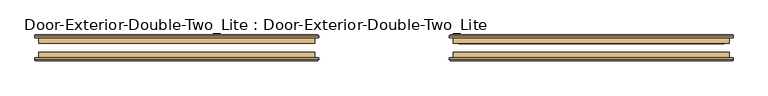
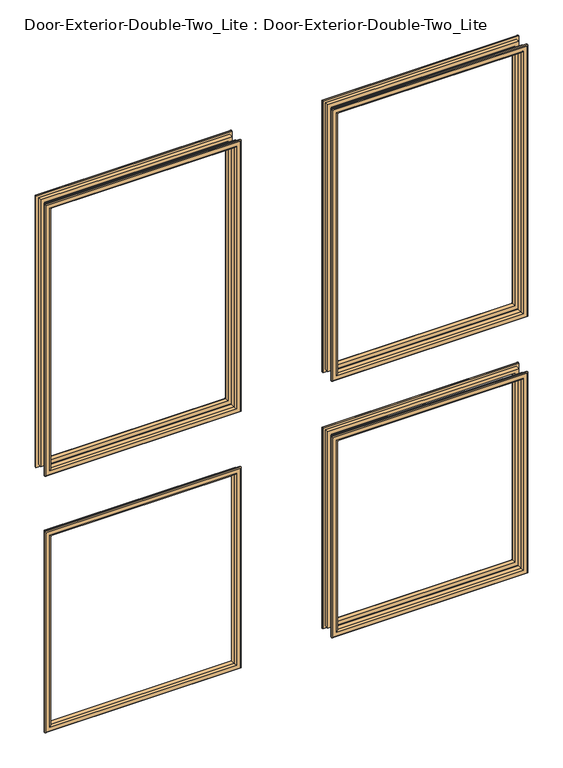
"""IFC4 building model written with IfcOpenShell, lengths in millimetres: door geometry, Door-Exterior-Double-Two_Lite : Door-Exterior-Double-Two_Lite."""

from ifc_helpers import new_model, si_unit, frame, origin, place, context, project, spatial, ellipse_curve, source, transform, mapped, element, save
from ifc_brep_helpers import plane_surface, cylinder_surface, advanced_brep


def door_exterior_double_two_lite_door_exterior_double_two_lite_6b883914(model_context):
    return source(origin(), model_context, "Body", "AdvancedBrep", [
        advanced_brep(
        [(-762.0, 99.2, 1117.6), (-762.0, 86.5, 1117.6), (-762.0, 86.5, 2016.125), (-762.0, 99.2, 2016.125), (-750.0, 85.5, 1129.6), (-750.0, 99.2, 1129.6), (-750.0, 99.2, 2004.125), (-750.0, 85.5, 2004.125), (-755.0, 80.5, 1124.6), (-755.0, 80.5, 2009.125), (-770.0, 82.5, 1109.6), (-768.0, 80.5, 1111.6), (-768.0, 80.5, 2022.125), (-770.0, 82.5, 2024.125), (-770.0, 86.5, 1109.6), (-770.0, 86.5, 2024.125), (-152.4, 86.5, 2016.125), (-152.4, 99.2, 2016.125), (-164.4, 99.2, 2004.125), (-164.4, 85.5, 2004.125), (-159.4, 80.5, 2009.125), (-146.4, 80.5, 2022.125), (-144.4, 82.5, 2024.125), (-144.4, 86.5, 2024.125), (-152.4, 86.5, 1117.6), (-152.4, 99.2, 1117.6), (-164.4, 99.2, 1129.6), (-164.4, 85.5, 1129.6), (-159.4, 80.5, 1124.6), (-146.4, 80.5, 1111.6), (-144.4, 82.5, 1109.6), (-144.4, 86.5, 1109.6)],
        [
            (0, 1),
            (1, 2),
            (2, 3),
            (3, 0),
            (4, 5),
            (5, 6),
            (6, 7),
            (7, 4),
            (8, 4, ellipse_curve(frame((-755.0, 85.5, 1124.6), z_axis=(-0.7071067811865475, 0.0, 0.7071067811865475), x_axis=(-0.7071067811865474, 0.0, -0.7071067811865476)), 7.0710678, 5.0)),
            (7, 9, ellipse_curve(frame((-755.0, 85.5, 2009.125), z_axis=(-0.7071067811865475, 0.0, -0.7071067811865475), x_axis=(0.7071067811865474, 0.0, -0.7071067811865476)), 7.0710678, 5.0)),
            (9, 8),
            (10, 11, ellipse_curve(frame((-768.0, 82.5, 1111.6), z_axis=(-0.7071067811865475, 0.0, 0.7071067811865475), x_axis=(-0.7071067811865474, 0.0, -0.7071067811865476)), 2.8284271, 2.0)),
            (11, 12),
            (12, 13, ellipse_curve(frame((-768.0, 82.5, 2022.125), z_axis=(-0.7071067811865475, 0.0, -0.7071067811865475), x_axis=(0.7071067811865474, 0.0, -0.7071067811865476)), 2.8284271, 2.0)),
            (13, 10),
            (14, 10),
            (13, 15),
            (15, 14),
            (2, 16),
            (16, 17),
            (17, 3),
            (6, 18),
            (18, 19),
            (19, 7),
            (19, 20, ellipse_curve(frame((-159.4, 85.5, 2009.125), z_axis=(-0.7071067811865475, 0.0, 0.7071067811865475), x_axis=(-0.7071067811865476, 0.0, -0.7071067811865474)), 7.0710678, 5.0)),
            (20, 9),
            (12, 21),
            (21, 22, ellipse_curve(frame((-146.4, 82.5, 2022.125), z_axis=(-0.7071067811865475, 0.0, 0.7071067811865475), x_axis=(-0.7071067811865476, 0.0, -0.7071067811865474)), 2.8284271, 2.0)),
            (22, 13),
            (22, 23),
            (23, 15),
            (16, 24),
            (24, 25),
            (25, 17),
            (18, 26),
            (26, 27),
            (27, 19),
            (27, 28, ellipse_curve(frame((-159.4, 85.5, 1124.6), z_axis=(0.7071067811865475, 0.0, 0.7071067811865475), x_axis=(-0.7071067811865474, 0.0, 0.7071067811865476)), 7.0710678, 5.0)),
            (28, 20),
            (21, 29),
            (29, 30, ellipse_curve(frame((-146.4, 82.5, 1111.6), z_axis=(0.7071067811865475, 0.0, 0.7071067811865475), x_axis=(-0.7071067811865474, 0.0, 0.7071067811865476)), 2.8284271, 2.0)),
            (30, 22),
            (30, 31),
            (31, 23),
            (31, 14),
            (1, 24),
            (0, 25),
            (5, 26),
            (4, 27),
            (8, 28),
            (11, 29),
            (10, 30),
        ],
        [
            plane_surface(frame((-762.0, 86.5, 1117.6), z_axis=(-1.0, 0.0, 0.0), x_axis=(0.0, 0.0, 1.0))),
            plane_surface(frame((-750.0, 99.2, 1129.6), z_axis=(1.0, 0.0, 0.0), x_axis=(0.0, 0.0, 1.0))),
            cylinder_surface(frame((-755.0, 85.5, 1117.6), z_axis=(0.0, 0.0, -1.0), x_axis=(-1.0, 0.0, 0.0)), 5.0),
            cylinder_surface(frame((-768.0, 82.5, 1117.6), z_axis=(0.0, 0.0, -1.0), x_axis=(-1.0, 0.0, 0.0)), 2.0),
            plane_surface(frame((-770.0, 82.5, 1109.6), z_axis=(-1.0, 0.0, 0.0), x_axis=(0.0, 0.0, 1.0))),
            plane_surface(frame((-762.0, 86.5, 2016.125), z_axis=(0.0, 0.0, 1.0), x_axis=(1.0, 0.0, 0.0))),
            plane_surface(frame((-750.0, 99.2, 2004.125), z_axis=(0.0, 0.0, -1.0), x_axis=(1.0, 0.0, 0.0))),
            cylinder_surface(frame((-762.0, 85.5, 2009.125), z_axis=(-1.0, 0.0, 0.0), x_axis=(0.0, 0.0, 1.0)), 5.0),
            cylinder_surface(frame((-762.0, 82.5, 2022.125), z_axis=(-1.0, 0.0, 0.0), x_axis=(0.0, 0.0, 1.0)), 2.0),
            plane_surface(frame((-770.0, 82.5, 2024.125), z_axis=(0.0, 0.0, 1.0), x_axis=(1.0, 0.0, 0.0))),
            plane_surface(frame((-152.4, 86.5, 2016.125), z_axis=(1.0, 0.0, 0.0), x_axis=(0.0, 0.0, -1.0))),
            plane_surface(frame((-164.4, 99.2, 2004.125), z_axis=(-1.0, 0.0, 0.0), x_axis=(0.0, 0.0, -1.0))),
            cylinder_surface(frame((-159.4, 85.5, 2016.125), z_axis=(0.0, 0.0, 1.0), x_axis=(1.0, 0.0, 0.0)), 5.0),
            cylinder_surface(frame((-146.4, 82.5, 2016.125), z_axis=(0.0, 0.0, 1.0), x_axis=(1.0, 0.0, 0.0)), 2.0),
            plane_surface(frame((-144.4, 82.5, 2024.125), z_axis=(1.0, 0.0, 0.0), x_axis=(0.0, 0.0, -1.0))),
            plane_surface(frame((-144.4, 86.5, 1109.6), z_axis=(0.0, 1.0, 0.0), x_axis=(-1.0, 0.0, 0.0))),
            plane_surface(frame((-152.4, 86.5, 1117.6), z_axis=(0.0, 0.0, -1.0), x_axis=(-1.0, 0.0, 0.0))),
            plane_surface(frame((-152.4, 99.2, 1117.6), z_axis=(0.0, 1.0, 0.0), x_axis=(-1.0, 0.0, 0.0))),
            plane_surface(frame((-164.4, 99.2, 1129.6), z_axis=(0.0, 0.0, 1.0), x_axis=(-1.0, 0.0, 0.0))),
            cylinder_surface(frame((-152.4, 85.5, 1124.6), z_axis=(1.0, 0.0, 0.0), x_axis=(0.0, 0.0, -1.0)), 5.0),
            plane_surface(frame((-159.4, 80.5, 1124.6), z_axis=(0.0, -1.0, 0.0), x_axis=(-1.0, 0.0, 0.0))),
            cylinder_surface(frame((-152.4, 82.5, 1111.6), z_axis=(1.0, 0.0, 0.0), x_axis=(0.0, 0.0, -1.0)), 2.0),
            plane_surface(frame((-144.4, 82.5, 1109.6), z_axis=(0.0, 0.0, -1.0), x_axis=(-1.0, 0.0, 0.0))),
        ],
        [
            (0, [[1, 2, 3, 4]]),
            (1, [[5, 6, 7, 8]]),
            (2, [[9, -8, 10, 11]]),
            (3, [[12, 13, 14, 15]]),
            (4, [[16, -15, 17, 18]]),
            (5, [[-3, 19, 20, 21]]),
            (6, [[-7, 22, 23, 24]]),
            (7, [[-10, -24, 25, 26]]),
            (8, [[-14, 27, 28, 29]]),
            (9, [[-17, -29, 30, 31]]),
            (10, [[-20, 32, 33, 34]]),
            (11, [[-23, 35, 36, 37]]),
            (12, [[-25, -37, 38, 39]]),
            (13, [[-28, 40, 41, 42]]),
            (14, [[-30, -42, 43, 44]]),
            (15, [[-31, -44, 45, -18], [46, -32, -19, -2]]),
            (16, [[-33, -46, -1, 47]]),
            (17, [[-21, -34, -47, -4], [48, -35, -22, -6]]),
            (18, [[-36, -48, -5, 49]]),
            (19, [[-38, -49, -9, 50]]),
            (20, [[51, -40, -27, -13], [-26, -39, -50, -11]]),
            (21, [[-41, -51, -12, 52]]),
            (22, [[-43, -52, -16, -45]]),
        ],
    ),
        advanced_brep(
        [(152.4, 99.2, 1117.6), (152.4, 86.5, 1117.6), (152.4, 86.5, 2016.125), (152.4, 99.2, 2016.125), (164.4, 85.5, 1129.6), (164.4, 99.2, 1129.6), (164.4, 99.2, 2004.125), (164.4, 85.5, 2004.125), (159.4, 80.5, 1124.6), (159.4, 80.5, 2009.125), (144.4, 82.5, 1109.6), (146.4, 80.5, 1111.6), (146.4, 80.5, 2022.125), (144.4, 82.5, 2024.125), (144.4, 86.5, 1109.6), (144.4, 86.5, 2024.125), (762.0, 86.5, 2016.125), (762.0, 99.2, 2016.125), (750.0, 99.2, 2004.125), (750.0, 85.5, 2004.125), (755.0, 80.5, 2009.125), (768.0, 80.5, 2022.125), (770.0, 82.5, 2024.125), (770.0, 86.5, 2024.125), (762.0, 86.5, 1117.6), (762.0, 99.2, 1117.6), (750.0, 99.2, 1129.6), (750.0, 85.5, 1129.6), (755.0, 80.5, 1124.6), (768.0, 80.5, 1111.6), (770.0, 82.5, 1109.6), (770.0, 86.5, 1109.6)],
        [
            (0, 1),
            (1, 2),
            (2, 3),
            (3, 0),
            (4, 5),
            (5, 6),
            (6, 7),
            (7, 4),
            (8, 4, ellipse_curve(frame((159.4, 85.5, 1124.6), z_axis=(-0.7071067811865475, 0.0, 0.7071067811865475), x_axis=(-0.7071067811865474, 0.0, -0.7071067811865476)), 7.0710678, 5.0)),
            (7, 9, ellipse_curve(frame((159.4, 85.5, 2009.125), z_axis=(-0.7071067811865475, 0.0, -0.7071067811865475), x_axis=(0.7071067811865474, 0.0, -0.7071067811865476)), 7.0710678, 5.0)),
            (9, 8),
            (10, 11, ellipse_curve(frame((146.4, 82.5, 1111.6), z_axis=(-0.7071067811865475, 0.0, 0.7071067811865475), x_axis=(-0.7071067811865474, 0.0, -0.7071067811865476)), 2.8284271, 2.0)),
            (11, 12),
            (12, 13, ellipse_curve(frame((146.4, 82.5, 2022.125), z_axis=(-0.7071067811865475, 0.0, -0.7071067811865475), x_axis=(0.7071067811865474, 0.0, -0.7071067811865476)), 2.8284271, 2.0)),
            (13, 10),
            (14, 10),
            (13, 15),
            (15, 14),
            (2, 16),
            (16, 17),
            (17, 3),
            (6, 18),
            (18, 19),
            (19, 7),
            (19, 20, ellipse_curve(frame((755.0, 85.5, 2009.125), z_axis=(-0.7071067811865475, 0.0, 0.7071067811865475), x_axis=(-0.7071067811865476, 0.0, -0.7071067811865474)), 7.0710678, 5.0)),
            (20, 9),
            (12, 21),
            (21, 22, ellipse_curve(frame((768.0, 82.5, 2022.125), z_axis=(-0.7071067811865475, 0.0, 0.7071067811865475), x_axis=(-0.7071067811865476, 0.0, -0.7071067811865474)), 2.8284271, 2.0)),
            (22, 13),
            (22, 23),
            (23, 15),
            (16, 24),
            (24, 25),
            (25, 17),
            (18, 26),
            (26, 27),
            (27, 19),
            (27, 28, ellipse_curve(frame((755.0, 85.5, 1124.6), z_axis=(0.7071067811865475, 0.0, 0.7071067811865475), x_axis=(-0.7071067811865474, 0.0, 0.7071067811865476)), 7.0710678, 5.0)),
            (28, 20),
            (21, 29),
            (29, 30, ellipse_curve(frame((768.0, 82.5, 1111.6), z_axis=(0.7071067811865475, 0.0, 0.7071067811865475), x_axis=(-0.7071067811865474, 0.0, 0.7071067811865476)), 2.8284271, 2.0)),
            (30, 22),
            (30, 31),
            (31, 23),
            (31, 14),
            (1, 24),
            (0, 25),
            (5, 26),
            (4, 27),
            (8, 28),
            (11, 29),
            (10, 30),
        ],
        [
            plane_surface(frame((152.4, 86.5, 1117.6), z_axis=(-1.0, 0.0, 0.0), x_axis=(0.0, 0.0, 1.0))),
            plane_surface(frame((164.4, 99.2, 1129.6), z_axis=(1.0, 0.0, 0.0), x_axis=(0.0, 0.0, 1.0))),
            cylinder_surface(frame((159.4, 85.5, 1117.6), z_axis=(0.0, 0.0, -1.0), x_axis=(-1.0, 0.0, 0.0)), 5.0),
            cylinder_surface(frame((146.4, 82.5, 1117.6), z_axis=(0.0, 0.0, -1.0), x_axis=(-1.0, 0.0, 0.0)), 2.0),
            plane_surface(frame((144.4, 82.5, 1109.6), z_axis=(-1.0, 0.0, 0.0), x_axis=(0.0, 0.0, 1.0))),
            plane_surface(frame((152.4, 86.5, 2016.125), z_axis=(0.0, 0.0, 1.0), x_axis=(1.0, 0.0, 0.0))),
            plane_surface(frame((164.4, 99.2, 2004.125), z_axis=(0.0, 0.0, -1.0), x_axis=(1.0, 0.0, 0.0))),
            cylinder_surface(frame((152.4, 85.5, 2009.125), z_axis=(-1.0, 0.0, 0.0), x_axis=(0.0, 0.0, 1.0)), 5.0),
            cylinder_surface(frame((152.4, 82.5, 2022.125), z_axis=(-1.0, 0.0, 0.0), x_axis=(0.0, 0.0, 1.0)), 2.0),
            plane_surface(frame((144.4, 82.5, 2024.125), z_axis=(0.0, 0.0, 1.0), x_axis=(1.0, 0.0, 0.0))),
            plane_surface(frame((762.0, 86.5, 2016.125), z_axis=(1.0, 0.0, 0.0), x_axis=(0.0, 0.0, -1.0))),
            plane_surface(frame((750.0, 99.2, 2004.125), z_axis=(-1.0, 0.0, 0.0), x_axis=(0.0, 0.0, -1.0))),
            cylinder_surface(frame((755.0, 85.5, 2016.125), z_axis=(0.0, 0.0, 1.0), x_axis=(1.0, 0.0, 0.0)), 5.0),
            cylinder_surface(frame((768.0, 82.5, 2016.125), z_axis=(0.0, 0.0, 1.0), x_axis=(1.0, 0.0, 0.0)), 2.0),
            plane_surface(frame((770.0, 82.5, 2024.125), z_axis=(1.0, 0.0, 0.0), x_axis=(0.0, 0.0, -1.0))),
            plane_surface(frame((770.0, 86.5, 1109.6), z_axis=(0.0, 1.0, 0.0), x_axis=(-1.0, 0.0, 0.0))),
            plane_surface(frame((762.0, 86.5, 1117.6), z_axis=(0.0, 0.0, -1.0), x_axis=(-1.0, 0.0, 0.0))),
            plane_surface(frame((762.0, 99.2, 1117.6), z_axis=(0.0, 1.0, 0.0), x_axis=(-1.0, 0.0, 0.0))),
            plane_surface(frame((750.0, 99.2, 1129.6), z_axis=(0.0, 0.0, 1.0), x_axis=(-1.0, 0.0, 0.0))),
            cylinder_surface(frame((762.0, 85.5, 1124.6), z_axis=(1.0, 0.0, 0.0), x_axis=(0.0, 0.0, -1.0)), 5.0),
            plane_surface(frame((755.0, 80.5, 1124.6), z_axis=(0.0, -1.0, 0.0), x_axis=(-1.0, 0.0, 0.0))),
            cylinder_surface(frame((762.0, 82.5, 1111.6), z_axis=(1.0, 0.0, 0.0), x_axis=(0.0, 0.0, -1.0)), 2.0),
            plane_surface(frame((770.0, 82.5, 1109.6), z_axis=(0.0, 0.0, -1.0), x_axis=(-1.0, 0.0, 0.0))),
        ],
        [
            (0, [[1, 2, 3, 4]]),
            (1, [[5, 6, 7, 8]]),
            (2, [[9, -8, 10, 11]]),
            (3, [[12, 13, 14, 15]]),
            (4, [[16, -15, 17, 18]]),
            (5, [[-3, 19, 20, 21]]),
            (6, [[-7, 22, 23, 24]]),
            (7, [[-10, -24, 25, 26]]),
            (8, [[-14, 27, 28, 29]]),
            (9, [[-17, -29, 30, 31]]),
            (10, [[-20, 32, 33, 34]]),
            (11, [[-23, 35, 36, 37]]),
            (12, [[-25, -37, 38, 39]]),
            (13, [[-28, 40, 41, 42]]),
            (14, [[-30, -42, 43, 44]]),
            (15, [[-31, -44, 45, -18], [46, -32, -19, -2]]),
            (16, [[-33, -46, -1, 47]]),
            (17, [[-21, -34, -47, -4], [48, -35, -22, -6]]),
            (18, [[-36, -48, -5, 49]]),
            (19, [[-38, -49, -9, 50]]),
            (20, [[51, -40, -27, -13], [-26, -39, -50, -11]]),
            (21, [[-41, -51, -12, 52]]),
            (22, [[-43, -52, -16, -45]]),
        ],
    ),
        advanced_brep(
        [(152.4, 99.2, 254.0), (152.4, 86.5, 254.0), (152.4, 86.5, 914.4), (152.4, 99.2, 914.4), (164.4, 85.5, 266.0), (164.4, 99.2, 266.0), (164.4, 99.2, 902.4), (164.4, 85.5, 902.4), (159.4, 80.5, 261.0), (159.4, 80.5, 907.4), (144.4, 82.5, 246.0), (146.4, 80.5, 248.0), (146.4, 80.5, 920.4), (144.4, 82.5, 922.4), (144.4, 86.5, 246.0), (144.4, 86.5, 922.4), (762.0, 86.5, 914.4), (762.0, 99.2, 914.4), (750.0, 99.2, 902.4), (750.0, 85.5, 902.4), (755.0, 80.5, 907.4), (768.0, 80.5, 920.4), (770.0, 82.5, 922.4), (770.0, 86.5, 922.4), (762.0, 86.5, 254.0), (762.0, 99.2, 254.0), (750.0, 99.2, 266.0), (750.0, 85.5, 266.0), (755.0, 80.5, 261.0), (768.0, 80.5, 248.0), (770.0, 82.5, 246.0), (770.0, 86.5, 246.0)],
        [
            (0, 1),
            (1, 2),
            (2, 3),
            (3, 0),
            (4, 5),
            (5, 6),
            (6, 7),
            (7, 4),
            (8, 4, ellipse_curve(frame((159.4, 85.5, 261.0), z_axis=(-0.7071067811865475, 0.0, 0.7071067811865475), x_axis=(-0.7071067811865474, 0.0, -0.7071067811865476)), 7.0710678, 5.0)),
            (7, 9, ellipse_curve(frame((159.4, 85.5, 907.4), z_axis=(-0.7071067811865475, 0.0, -0.7071067811865475), x_axis=(0.7071067811865474, 0.0, -0.7071067811865476)), 7.0710678, 5.0)),
            (9, 8),
            (10, 11, ellipse_curve(frame((146.4, 82.5, 248.0), z_axis=(-0.7071067811865475, 0.0, 0.7071067811865475), x_axis=(-0.7071067811865474, 0.0, -0.7071067811865476)), 2.8284271, 2.0)),
            (11, 12),
            (12, 13, ellipse_curve(frame((146.4, 82.5, 920.4), z_axis=(-0.7071067811865475, 0.0, -0.7071067811865475), x_axis=(0.7071067811865474, 0.0, -0.7071067811865476)), 2.8284271, 2.0)),
            (13, 10),
            (14, 10),
            (13, 15),
            (15, 14),
            (2, 16),
            (16, 17),
            (17, 3),
            (6, 18),
            (18, 19),
            (19, 7),
            (19, 20, ellipse_curve(frame((755.0, 85.5, 907.4), z_axis=(-0.7071067811865475, 0.0, 0.7071067811865475), x_axis=(-0.7071067811865476, 0.0, -0.7071067811865474)), 7.0710678, 5.0)),
            (20, 9),
            (12, 21),
            (21, 22, ellipse_curve(frame((768.0, 82.5, 920.4), z_axis=(-0.7071067811865475, 0.0, 0.7071067811865475), x_axis=(-0.7071067811865476, 0.0, -0.7071067811865474)), 2.8284271, 2.0)),
            (22, 13),
            (22, 23),
            (23, 15),
            (16, 24),
            (24, 25),
            (25, 17),
            (18, 26),
            (26, 27),
            (27, 19),
            (27, 28, ellipse_curve(frame((755.0, 85.5, 261.0), z_axis=(0.7071067811865475, 0.0, 0.7071067811865475), x_axis=(-0.7071067811865474, 0.0, 0.7071067811865476)), 7.0710678, 5.0)),
            (28, 20),
            (21, 29),
            (29, 30, ellipse_curve(frame((768.0, 82.5, 248.0), z_axis=(0.7071067811865475, 0.0, 0.7071067811865475), x_axis=(-0.7071067811865474, 0.0, 0.7071067811865476)), 2.8284271, 2.0)),
            (30, 22),
            (30, 31),
            (31, 23),
            (31, 14),
            (1, 24),
            (0, 25),
            (5, 26),
            (4, 27),
            (8, 28),
            (11, 29),
            (10, 30),
        ],
        [
            plane_surface(frame((152.4, 86.5, 254.0), z_axis=(-1.0, 0.0, 0.0), x_axis=(0.0, 0.0, 1.0))),
            plane_surface(frame((164.4, 99.2, 266.0), z_axis=(1.0, 0.0, 0.0), x_axis=(0.0, 0.0, 1.0))),
            cylinder_surface(frame((159.4, 85.5, 254.0), z_axis=(0.0, 0.0, -1.0), x_axis=(-1.0, 0.0, 0.0)), 5.0),
            cylinder_surface(frame((146.4, 82.5, 254.0), z_axis=(0.0, 0.0, -1.0), x_axis=(-1.0, 0.0, 0.0)), 2.0),
            plane_surface(frame((144.4, 82.5, 246.0), z_axis=(-1.0, 0.0, 0.0), x_axis=(0.0, 0.0, 1.0))),
            plane_surface(frame((152.4, 86.5, 914.4), z_axis=(0.0, 0.0, 1.0), x_axis=(1.0, 0.0, 0.0))),
            plane_surface(frame((164.4, 99.2, 902.4), z_axis=(0.0, 0.0, -1.0), x_axis=(1.0, 0.0, 0.0))),
            cylinder_surface(frame((152.4, 85.5, 907.4), z_axis=(-1.0, 0.0, 0.0), x_axis=(0.0, 0.0, 1.0)), 5.0),
            cylinder_surface(frame((152.4, 82.5, 920.4), z_axis=(-1.0, 0.0, 0.0), x_axis=(0.0, 0.0, 1.0)), 2.0),
            plane_surface(frame((144.4, 82.5, 922.4), z_axis=(0.0, 0.0, 1.0), x_axis=(1.0, 0.0, 0.0))),
            plane_surface(frame((762.0, 86.5, 914.4), z_axis=(1.0, 0.0, 0.0), x_axis=(0.0, 0.0, -1.0))),
            plane_surface(frame((750.0, 99.2, 902.4), z_axis=(-1.0, 0.0, 0.0), x_axis=(0.0, 0.0, -1.0))),
            cylinder_surface(frame((755.0, 85.5, 914.4), z_axis=(0.0, 0.0, 1.0), x_axis=(1.0, 0.0, 0.0)), 5.0),
            cylinder_surface(frame((768.0, 82.5, 914.4), z_axis=(0.0, 0.0, 1.0), x_axis=(1.0, 0.0, 0.0)), 2.0),
            plane_surface(frame((770.0, 82.5, 922.4), z_axis=(1.0, 0.0, 0.0), x_axis=(0.0, 0.0, -1.0))),
            plane_surface(frame((770.0, 86.5, 246.0), z_axis=(0.0, 1.0, 0.0), x_axis=(-1.0, 0.0, 0.0))),
            plane_surface(frame((762.0, 86.5, 254.0), z_axis=(0.0, 0.0, -1.0), x_axis=(-1.0, 0.0, 0.0))),
            plane_surface(frame((762.0, 99.2, 254.0), z_axis=(0.0, 1.0, 0.0), x_axis=(-1.0, 0.0, 0.0))),
            plane_surface(frame((750.0, 99.2, 266.0), z_axis=(0.0, 0.0, 1.0), x_axis=(-1.0, 0.0, 0.0))),
            cylinder_surface(frame((762.0, 85.5, 261.0), z_axis=(1.0, 0.0, 0.0), x_axis=(0.0, 0.0, -1.0)), 5.0),
            plane_surface(frame((755.0, 80.5, 261.0), z_axis=(0.0, -1.0, 0.0), x_axis=(-1.0, 0.0, 0.0))),
            cylinder_surface(frame((762.0, 82.5, 248.0), z_axis=(1.0, 0.0, 0.0), x_axis=(0.0, 0.0, -1.0)), 2.0),
            plane_surface(frame((770.0, 82.5, 246.0), z_axis=(0.0, 0.0, -1.0), x_axis=(-1.0, 0.0, 0.0))),
        ],
        [
            (0, [[1, 2, 3, 4]]),
            (1, [[5, 6, 7, 8]]),
            (2, [[9, -8, 10, 11]]),
            (3, [[12, 13, 14, 15]]),
            (4, [[16, -15, 17, 18]]),
            (5, [[-3, 19, 20, 21]]),
            (6, [[-7, 22, 23, 24]]),
            (7, [[-10, -24, 25, 26]]),
            (8, [[-14, 27, 28, 29]]),
            (9, [[-17, -29, 30, 31]]),
            (10, [[-20, 32, 33, 34]]),
            (11, [[-23, 35, 36, 37]]),
            (12, [[-25, -37, 38, 39]]),
            (13, [[-28, 40, 41, 42]]),
            (14, [[-30, -42, 43, 44]]),
            (15, [[-31, -44, 45, -18], [46, -32, -19, -2]]),
            (16, [[-33, -46, -1, 47]]),
            (17, [[-21, -34, -47, -4], [48, -35, -22, -6]]),
            (18, [[-36, -48, -5, 49]]),
            (19, [[-38, -49, -9, 50]]),
            (20, [[51, -40, -27, -13], [-26, -39, -50, -11]]),
            (21, [[-41, -51, -12, 52]]),
            (22, [[-43, -52, -16, -45]]),
        ],
    ),
        advanced_brep(
        [(-762.0, 99.2, 254.0), (-762.0, 86.5, 254.0), (-762.0, 86.5, 914.4), (-762.0, 99.2, 914.4), (-750.0, 85.5, 266.0), (-750.0, 99.2, 266.0), (-750.0, 99.2, 902.4), (-750.0, 85.5, 902.4), (-755.0, 80.5, 261.0), (-755.0, 80.5, 907.4), (-770.0, 82.5, 246.0), (-768.0, 80.5, 248.0), (-768.0, 80.5, 920.4), (-770.0, 82.5, 922.4), (-770.0, 86.5, 246.0), (-770.0, 86.5, 922.4), (-152.4, 86.5, 914.4), (-152.4, 99.2, 914.4), (-164.4, 99.2, 902.4), (-164.4, 85.5, 902.4), (-159.4, 80.5, 907.4), (-146.4, 80.5, 920.4), (-144.4, 82.5, 922.4), (-144.4, 86.5, 922.4), (-152.4, 86.5, 254.0), (-152.4, 99.2, 254.0), (-164.4, 99.2, 266.0), (-164.4, 85.5, 266.0), (-159.4, 80.5, 261.0), (-146.4, 80.5, 248.0), (-144.4, 82.5, 246.0), (-144.4, 86.5, 246.0)],
        [
            (0, 1),
            (1, 2),
            (2, 3),
            (3, 0),
            (4, 5),
            (5, 6),
            (6, 7),
            (7, 4),
            (8, 4, ellipse_curve(frame((-755.0, 85.5, 261.0), z_axis=(-0.7071067811865475, 0.0, 0.7071067811865475), x_axis=(-0.7071067811865474, 0.0, -0.7071067811865476)), 7.0710678, 5.0)),
            (7, 9, ellipse_curve(frame((-755.0, 85.5, 907.4), z_axis=(-0.7071067811865475, 0.0, -0.7071067811865475), x_axis=(0.7071067811865474, 0.0, -0.7071067811865476)), 7.0710678, 5.0)),
            (9, 8),
            (10, 11, ellipse_curve(frame((-768.0, 82.5, 248.0), z_axis=(-0.7071067811865475, 0.0, 0.7071067811865475), x_axis=(-0.7071067811865474, 0.0, -0.7071067811865476)), 2.8284271, 2.0)),
            (11, 12),
            (12, 13, ellipse_curve(frame((-768.0, 82.5, 920.4), z_axis=(-0.7071067811865475, 0.0, -0.7071067811865475), x_axis=(0.7071067811865474, 0.0, -0.7071067811865476)), 2.8284271, 2.0)),
            (13, 10),
            (14, 10),
            (13, 15),
            (15, 14),
            (2, 16),
            (16, 17),
            (17, 3),
            (6, 18),
            (18, 19),
            (19, 7),
            (19, 20, ellipse_curve(frame((-159.4, 85.5, 907.4), z_axis=(-0.7071067811865475, 0.0, 0.7071067811865475), x_axis=(-0.7071067811865476, 0.0, -0.7071067811865474)), 7.0710678, 5.0)),
            (20, 9),
            (12, 21),
            (21, 22, ellipse_curve(frame((-146.4, 82.5, 920.4), z_axis=(-0.7071067811865475, 0.0, 0.7071067811865475), x_axis=(-0.7071067811865476, 0.0, -0.7071067811865474)), 2.8284271, 2.0)),
            (22, 13),
            (22, 23),
            (23, 15),
            (16, 24),
            (24, 25),
            (25, 17),
            (18, 26),
            (26, 27),
            (27, 19),
            (27, 28, ellipse_curve(frame((-159.4, 85.5, 261.0), z_axis=(0.7071067811865475, 0.0, 0.7071067811865475), x_axis=(-0.7071067811865474, 0.0, 0.7071067811865476)), 7.0710678, 5.0)),
            (28, 20),
            (21, 29),
            (29, 30, ellipse_curve(frame((-146.4, 82.5, 248.0), z_axis=(0.7071067811865475, 0.0, 0.7071067811865475), x_axis=(-0.7071067811865474, 0.0, 0.7071067811865476)), 2.8284271, 2.0)),
            (30, 22),
            (30, 31),
            (31, 23),
            (31, 14),
            (1, 24),
            (0, 25),
            (5, 26),
            (4, 27),
            (8, 28),
            (11, 29),
            (10, 30),
        ],
        [
            plane_surface(frame((-762.0, 86.5, 254.0), z_axis=(-1.0, 0.0, 0.0), x_axis=(0.0, 0.0, 1.0))),
            plane_surface(frame((-750.0, 99.2, 266.0), z_axis=(1.0, 0.0, 0.0), x_axis=(0.0, 0.0, 1.0))),
            cylinder_surface(frame((-755.0, 85.5, 254.0), z_axis=(0.0, 0.0, -1.0), x_axis=(-1.0, 0.0, 0.0)), 5.0),
            cylinder_surface(frame((-768.0, 82.5, 254.0), z_axis=(0.0, 0.0, -1.0), x_axis=(-1.0, 0.0, 0.0)), 2.0),
            plane_surface(frame((-770.0, 82.5, 246.0), z_axis=(-1.0, 0.0, 0.0), x_axis=(0.0, 0.0, 1.0))),
            plane_surface(frame((-762.0, 86.5, 914.4), z_axis=(0.0, 0.0, 1.0), x_axis=(1.0, 0.0, 0.0))),
            plane_surface(frame((-750.0, 99.2, 902.4), z_axis=(0.0, 0.0, -1.0), x_axis=(1.0, 0.0, 0.0))),
            cylinder_surface(frame((-762.0, 85.5, 907.4), z_axis=(-1.0, 0.0, 0.0), x_axis=(0.0, 0.0, 1.0)), 5.0),
            cylinder_surface(frame((-762.0, 82.5, 920.4), z_axis=(-1.0, 0.0, 0.0), x_axis=(0.0, 0.0, 1.0)), 2.0),
            plane_surface(frame((-770.0, 82.5, 922.4), z_axis=(0.0, 0.0, 1.0), x_axis=(1.0, 0.0, 0.0))),
            plane_surface(frame((-152.4, 86.5, 914.4), z_axis=(1.0, 0.0, 0.0), x_axis=(0.0, 0.0, -1.0))),
            plane_surface(frame((-164.4, 99.2, 902.4), z_axis=(-1.0, 0.0, 0.0), x_axis=(0.0, 0.0, -1.0))),
            cylinder_surface(frame((-159.4, 85.5, 914.4), z_axis=(0.0, 0.0, 1.0), x_axis=(1.0, 0.0, 0.0)), 5.0),
            cylinder_surface(frame((-146.4, 82.5, 914.4), z_axis=(0.0, 0.0, 1.0), x_axis=(1.0, 0.0, 0.0)), 2.0),
            plane_surface(frame((-144.4, 82.5, 922.4), z_axis=(1.0, 0.0, 0.0), x_axis=(0.0, 0.0, -1.0))),
            plane_surface(frame((-144.4, 86.5, 246.0), z_axis=(0.0, 1.0, 0.0), x_axis=(-1.0, 0.0, 0.0))),
            plane_surface(frame((-152.4, 86.5, 254.0), z_axis=(0.0, 0.0, -1.0), x_axis=(-1.0, 0.0, 0.0))),
            plane_surface(frame((-152.4, 99.2, 254.0), z_axis=(0.0, 1.0, 0.0), x_axis=(-1.0, 0.0, 0.0))),
            plane_surface(frame((-164.4, 99.2, 266.0), z_axis=(0.0, 0.0, 1.0), x_axis=(-1.0, 0.0, 0.0))),
            cylinder_surface(frame((-152.4, 85.5, 261.0), z_axis=(1.0, 0.0, 0.0), x_axis=(0.0, 0.0, -1.0)), 5.0),
            plane_surface(frame((-159.4, 80.5, 261.0), z_axis=(0.0, -1.0, 0.0), x_axis=(-1.0, 0.0, 0.0))),
            cylinder_surface(frame((-152.4, 82.5, 248.0), z_axis=(1.0, 0.0, 0.0), x_axis=(0.0, 0.0, -1.0)), 2.0),
            plane_surface(frame((-144.4, 82.5, 246.0), z_axis=(0.0, 0.0, -1.0), x_axis=(-1.0, 0.0, 0.0))),
        ],
        [
            (0, [[1, 2, 3, 4]]),
            (1, [[5, 6, 7, 8]]),
            (2, [[9, -8, 10, 11]]),
            (3, [[12, 13, 14, 15]]),
            (4, [[16, -15, 17, 18]]),
            (5, [[-3, 19, 20, 21]]),
            (6, [[-7, 22, 23, 24]]),
            (7, [[-10, -24, 25, 26]]),
            (8, [[-14, 27, 28, 29]]),
            (9, [[-17, -29, 30, 31]]),
            (10, [[-20, 32, 33, 34]]),
            (11, [[-23, 35, 36, 37]]),
            (12, [[-25, -37, 38, 39]]),
            (13, [[-28, 40, 41, 42]]),
            (14, [[-30, -42, 43, 44]]),
            (15, [[-31, -44, 45, -18], [46, -32, -19, -2]]),
            (16, [[-33, -46, -1, 47]]),
            (17, [[-21, -34, -47, -4], [48, -35, -22, -6]]),
            (18, [[-36, -48, -5, 49]]),
            (19, [[-38, -49, -9, 50]]),
            (20, [[51, -40, -27, -13], [-26, -39, -50, -11]]),
            (21, [[-41, -51, -12, 52]]),
            (22, [[-43, -52, -16, -45]]),
        ],
    ),
        advanced_brep(
        [(-762.0, 118.25, 2016.125), (-762.0, 130.95, 2016.125), (-762.0, 130.95, 1117.6), (-762.0, 118.25, 1117.6), (-750.0, 131.95, 2004.125), (-750.0, 118.25, 2004.125), (-750.0, 118.25, 1129.6), (-750.0, 131.95, 1129.6), (-755.0, 136.95, 2009.125), (-755.0, 136.95, 1124.6), (-770.0, 134.95, 2024.125), (-768.0, 136.95, 2022.125), (-768.0, 136.95, 1111.6), (-770.0, 134.95, 1109.6), (-770.0, 130.95, 2024.125), (-770.0, 130.95, 1109.6), (-152.4, 130.95, 1117.6), (-152.4, 118.25, 1117.6), (-164.4, 118.25, 1129.6), (-164.4, 131.95, 1129.6), (-159.4, 136.95, 1124.6), (-146.4, 136.95, 1111.6), (-144.4, 134.95, 1109.6), (-144.4, 130.95, 1109.6), (-152.4, 130.95, 2016.125), (-152.4, 118.25, 2016.125), (-164.4, 118.25, 2004.125), (-164.4, 131.95, 2004.125), (-159.4, 136.95, 2009.125), (-146.4, 136.95, 2022.125), (-144.4, 134.95, 2024.125), (-144.4, 130.95, 2024.125)],
        [
            (0, 1),
            (1, 2),
            (2, 3),
            (3, 0),
            (4, 5),
            (5, 6),
            (6, 7),
            (7, 4),
            (8, 4, ellipse_curve(frame((-755.0, 131.95, 2009.125), z_axis=(-0.7071067811865475, 0.0, -0.7071067811865475), x_axis=(-0.7071067811865474, 0.0, 0.7071067811865476)), 7.0710678, 5.0)),
            (7, 9, ellipse_curve(frame((-755.0, 131.95, 1124.6), z_axis=(-0.7071067811865475, 0.0, 0.7071067811865475), x_axis=(0.7071067811865474, 0.0, 0.7071067811865476)), 7.0710678, 5.0)),
            (9, 8),
            (10, 11, ellipse_curve(frame((-768.0, 134.95, 2022.125), z_axis=(-0.7071067811865475, 0.0, -0.7071067811865475), x_axis=(-0.7071067811865474, 0.0, 0.7071067811865476)), 2.8284271, 2.0)),
            (11, 12),
            (12, 13, ellipse_curve(frame((-768.0, 134.95, 1111.6), z_axis=(-0.7071067811865475, 0.0, 0.7071067811865475), x_axis=(0.7071067811865474, 0.0, 0.7071067811865476)), 2.8284271, 2.0)),
            (13, 10),
            (14, 10),
            (13, 15),
            (15, 14),
            (2, 16),
            (16, 17),
            (17, 3),
            (6, 18),
            (18, 19),
            (19, 7),
            (19, 20, ellipse_curve(frame((-159.4, 131.95, 1124.6), z_axis=(-0.7071067811865475, 0.0, -0.7071067811865475), x_axis=(-0.7071067811865476, 0.0, 0.7071067811865474)), 7.0710678, 5.0)),
            (20, 9),
            (12, 21),
            (21, 22, ellipse_curve(frame((-146.4, 134.95, 1111.6), z_axis=(-0.7071067811865475, 0.0, -0.7071067811865475), x_axis=(-0.7071067811865476, 0.0, 0.7071067811865474)), 2.8284271, 2.0)),
            (22, 13),
            (22, 23),
            (23, 15),
            (16, 24),
            (24, 25),
            (25, 17),
            (18, 26),
            (26, 27),
            (27, 19),
            (27, 28, ellipse_curve(frame((-159.4, 131.95, 2009.125), z_axis=(0.7071067811865475, 0.0, -0.7071067811865475), x_axis=(-0.7071067811865474, 0.0, -0.7071067811865476)), 7.0710678, 5.0)),
            (28, 20),
            (21, 29),
            (29, 30, ellipse_curve(frame((-146.4, 134.95, 2022.125), z_axis=(0.7071067811865475, 0.0, -0.7071067811865475), x_axis=(-0.7071067811865474, 0.0, -0.7071067811865476)), 2.8284271, 2.0)),
            (30, 22),
            (30, 31),
            (31, 23),
            (31, 14),
            (1, 24),
            (0, 25),
            (5, 26),
            (4, 27),
            (8, 28),
            (11, 29),
            (10, 30),
        ],
        [
            plane_surface(frame((-762.0, 130.95, 2016.125), z_axis=(-1.0, 0.0, 0.0), x_axis=(0.0, 0.0, -1.0))),
            plane_surface(frame((-750.0, 118.25, 2004.125), z_axis=(1.0, 0.0, 0.0), x_axis=(0.0, 0.0, -1.0))),
            cylinder_surface(frame((-755.0, 131.95, 2016.125), z_axis=(0.0, 0.0, 1.0), x_axis=(-1.0, 0.0, 0.0)), 5.0),
            cylinder_surface(frame((-768.0, 134.95, 2016.125), z_axis=(0.0, 0.0, 1.0), x_axis=(-1.0, 0.0, 0.0)), 2.0),
            plane_surface(frame((-770.0, 134.95, 2024.125), z_axis=(-1.0, 0.0, 0.0), x_axis=(0.0, 0.0, -1.0))),
            plane_surface(frame((-762.0, 130.95, 1117.6), z_axis=(0.0, 0.0, -1.0), x_axis=(1.0, 0.0, 0.0))),
            plane_surface(frame((-750.0, 118.25, 1129.6), z_axis=(0.0, 0.0, 1.0), x_axis=(1.0, 0.0, 0.0))),
            cylinder_surface(frame((-762.0, 131.95, 1124.6), z_axis=(-1.0, 0.0, 0.0), x_axis=(0.0, 0.0, -1.0)), 5.0),
            cylinder_surface(frame((-762.0, 134.95, 1111.6), z_axis=(-1.0, 0.0, 0.0), x_axis=(0.0, 0.0, -1.0)), 2.0),
            plane_surface(frame((-770.0, 134.95, 1109.6), z_axis=(0.0, 0.0, -1.0), x_axis=(1.0, 0.0, 0.0))),
            plane_surface(frame((-152.4, 130.95, 1117.6), z_axis=(1.0, 0.0, 0.0), x_axis=(0.0, 0.0, 1.0))),
            plane_surface(frame((-164.4, 118.25, 1129.6), z_axis=(-1.0, 0.0, 0.0), x_axis=(0.0, 0.0, 1.0))),
            cylinder_surface(frame((-159.4, 131.95, 1117.6), z_axis=(0.0, 0.0, -1.0), x_axis=(1.0, 0.0, 0.0)), 5.0),
            cylinder_surface(frame((-146.4, 134.95, 1117.6), z_axis=(0.0, 0.0, -1.0), x_axis=(1.0, 0.0, 0.0)), 2.0),
            plane_surface(frame((-144.4, 134.95, 1109.6), z_axis=(1.0, 0.0, 0.0), x_axis=(0.0, 0.0, 1.0))),
            plane_surface(frame((-144.4, 130.95, 2024.125), z_axis=(0.0, -1.0, 0.0), x_axis=(-1.0, 0.0, 0.0))),
            plane_surface(frame((-152.4, 130.95, 2016.125), z_axis=(0.0, 0.0, 1.0), x_axis=(-1.0, 0.0, 0.0))),
            plane_surface(frame((-152.4, 118.25, 2016.125), z_axis=(0.0, -1.0, 0.0), x_axis=(-1.0, 0.0, 0.0))),
            plane_surface(frame((-164.4, 118.25, 2004.125), z_axis=(0.0, 0.0, -1.0), x_axis=(-1.0, 0.0, 0.0))),
            cylinder_surface(frame((-152.4, 131.95, 2009.125), z_axis=(1.0, 0.0, 0.0), x_axis=(0.0, 0.0, 1.0)), 5.0),
            plane_surface(frame((-159.4, 136.95, 2009.125), z_axis=(0.0, 1.0, 0.0), x_axis=(-1.0, 0.0, 0.0))),
            cylinder_surface(frame((-152.4, 134.95, 2022.125), z_axis=(1.0, 0.0, 0.0), x_axis=(0.0, 0.0, 1.0)), 2.0),
            plane_surface(frame((-144.4, 134.95, 2024.125), z_axis=(0.0, 0.0, 1.0), x_axis=(-1.0, 0.0, 0.0))),
        ],
        [
            (0, [[1, 2, 3, 4]]),
            (1, [[5, 6, 7, 8]]),
            (2, [[9, -8, 10, 11]]),
            (3, [[12, 13, 14, 15]]),
            (4, [[16, -15, 17, 18]]),
            (5, [[-3, 19, 20, 21]]),
            (6, [[-7, 22, 23, 24]]),
            (7, [[-10, -24, 25, 26]]),
            (8, [[-14, 27, 28, 29]]),
            (9, [[-17, -29, 30, 31]]),
            (10, [[-20, 32, 33, 34]]),
            (11, [[-23, 35, 36, 37]]),
            (12, [[-25, -37, 38, 39]]),
            (13, [[-28, 40, 41, 42]]),
            (14, [[-30, -42, 43, 44]]),
            (15, [[-31, -44, 45, -18], [46, -32, -19, -2]]),
            (16, [[-33, -46, -1, 47]]),
            (17, [[-21, -34, -47, -4], [48, -35, -22, -6]]),
            (18, [[-36, -48, -5, 49]]),
            (19, [[-38, -49, -9, 50]]),
            (20, [[51, -40, -27, -13], [-26, -39, -50, -11]]),
            (21, [[-41, -51, -12, 52]]),
            (22, [[-43, -52, -16, -45]]),
        ],
    ),
        advanced_brep(
        [(152.4, 118.25, 2016.125), (152.4, 130.95, 2016.125), (152.4, 130.95, 1117.6), (152.4, 118.25, 1117.6), (164.4, 131.95, 2004.125), (164.4, 118.25, 2004.125), (164.4, 118.25, 1129.6), (164.4, 131.95, 1129.6), (159.4, 136.95, 2009.125), (159.4, 136.95, 1124.6), (144.4, 134.95, 2024.125), (146.4, 136.95, 2022.125), (146.4, 136.95, 1111.6), (144.4, 134.95, 1109.6), (144.4, 130.95, 2024.125), (144.4, 130.95, 1109.6), (762.0, 130.95, 1117.6), (762.0, 118.25, 1117.6), (750.0, 118.25, 1129.6), (750.0, 131.95, 1129.6), (755.0, 136.95, 1124.6), (768.0, 136.95, 1111.6), (770.0, 134.95, 1109.6), (770.0, 130.95, 1109.6), (762.0, 130.95, 2016.125), (762.0, 118.25, 2016.125), (750.0, 118.25, 2004.125), (750.0, 131.95, 2004.125), (755.0, 136.95, 2009.125), (768.0, 136.95, 2022.125), (770.0, 134.95, 2024.125), (770.0, 130.95, 2024.125)],
        [
            (0, 1),
            (1, 2),
            (2, 3),
            (3, 0),
            (4, 5),
            (5, 6),
            (6, 7),
            (7, 4),
            (8, 4, ellipse_curve(frame((159.4, 131.95, 2009.125), z_axis=(-0.7071067811865475, 0.0, -0.7071067811865475), x_axis=(-0.7071067811865474, 0.0, 0.7071067811865476)), 7.0710678, 5.0)),
            (7, 9, ellipse_curve(frame((159.4, 131.95, 1124.6), z_axis=(-0.7071067811865475, 0.0, 0.7071067811865475), x_axis=(0.7071067811865474, 0.0, 0.7071067811865476)), 7.0710678, 5.0)),
            (9, 8),
            (10, 11, ellipse_curve(frame((146.4, 134.95, 2022.125), z_axis=(-0.7071067811865475, 0.0, -0.7071067811865475), x_axis=(-0.7071067811865474, 0.0, 0.7071067811865476)), 2.8284271, 2.0)),
            (11, 12),
            (12, 13, ellipse_curve(frame((146.4, 134.95, 1111.6), z_axis=(-0.7071067811865475, 0.0, 0.7071067811865475), x_axis=(0.7071067811865474, 0.0, 0.7071067811865476)), 2.8284271, 2.0)),
            (13, 10),
            (14, 10),
            (13, 15),
            (15, 14),
            (2, 16),
            (16, 17),
            (17, 3),
            (6, 18),
            (18, 19),
            (19, 7),
            (19, 20, ellipse_curve(frame((755.0, 131.95, 1124.6), z_axis=(-0.7071067811865475, 0.0, -0.7071067811865475), x_axis=(-0.7071067811865476, 0.0, 0.7071067811865474)), 7.0710678, 5.0)),
            (20, 9),
            (12, 21),
            (21, 22, ellipse_curve(frame((768.0, 134.95, 1111.6), z_axis=(-0.7071067811865475, 0.0, -0.7071067811865475), x_axis=(-0.7071067811865476, 0.0, 0.7071067811865474)), 2.8284271, 2.0)),
            (22, 13),
            (22, 23),
            (23, 15),
            (16, 24),
            (24, 25),
            (25, 17),
            (18, 26),
            (26, 27),
            (27, 19),
            (27, 28, ellipse_curve(frame((755.0, 131.95, 2009.125), z_axis=(0.7071067811865475, 0.0, -0.7071067811865475), x_axis=(-0.7071067811865474, 0.0, -0.7071067811865476)), 7.0710678, 5.0)),
            (28, 20),
            (21, 29),
            (29, 30, ellipse_curve(frame((768.0, 134.95, 2022.125), z_axis=(0.7071067811865475, 0.0, -0.7071067811865475), x_axis=(-0.7071067811865474, 0.0, -0.7071067811865476)), 2.8284271, 2.0)),
            (30, 22),
            (30, 31),
            (31, 23),
            (31, 14),
            (1, 24),
            (0, 25),
            (5, 26),
            (4, 27),
            (8, 28),
            (11, 29),
            (10, 30),
        ],
        [
            plane_surface(frame((152.4, 130.95, 2016.125), z_axis=(-1.0, 0.0, 0.0), x_axis=(0.0, 0.0, -1.0))),
            plane_surface(frame((164.4, 118.25, 2004.125), z_axis=(1.0, 0.0, 0.0), x_axis=(0.0, 0.0, -1.0))),
            cylinder_surface(frame((159.4, 131.95, 2016.125), z_axis=(0.0, 0.0, 1.0), x_axis=(-1.0, 0.0, 0.0)), 5.0),
            cylinder_surface(frame((146.4, 134.95, 2016.125), z_axis=(0.0, 0.0, 1.0), x_axis=(-1.0, 0.0, 0.0)), 2.0),
            plane_surface(frame((144.4, 134.95, 2024.125), z_axis=(-1.0, 0.0, 0.0), x_axis=(0.0, 0.0, -1.0))),
            plane_surface(frame((152.4, 130.95, 1117.6), z_axis=(0.0, 0.0, -1.0), x_axis=(1.0, 0.0, 0.0))),
            plane_surface(frame((164.4, 118.25, 1129.6), z_axis=(0.0, 0.0, 1.0), x_axis=(1.0, 0.0, 0.0))),
            cylinder_surface(frame((152.4, 131.95, 1124.6), z_axis=(-1.0, 0.0, 0.0), x_axis=(0.0, 0.0, -1.0)), 5.0),
            cylinder_surface(frame((152.4, 134.95, 1111.6), z_axis=(-1.0, 0.0, 0.0), x_axis=(0.0, 0.0, -1.0)), 2.0),
            plane_surface(frame((144.4, 134.95, 1109.6), z_axis=(0.0, 0.0, -1.0), x_axis=(1.0, 0.0, 0.0))),
            plane_surface(frame((762.0, 130.95, 1117.6), z_axis=(1.0, 0.0, 0.0), x_axis=(0.0, 0.0, 1.0))),
            plane_surface(frame((750.0, 118.25, 1129.6), z_axis=(-1.0, 0.0, 0.0), x_axis=(0.0, 0.0, 1.0))),
            cylinder_surface(frame((755.0, 131.95, 1117.6), z_axis=(0.0, 0.0, -1.0), x_axis=(1.0, 0.0, 0.0)), 5.0),
            cylinder_surface(frame((768.0, 134.95, 1117.6), z_axis=(0.0, 0.0, -1.0), x_axis=(1.0, 0.0, 0.0)), 2.0),
            plane_surface(frame((770.0, 134.95, 1109.6), z_axis=(1.0, 0.0, 0.0), x_axis=(0.0, 0.0, 1.0))),
            plane_surface(frame((770.0, 130.95, 2024.125), z_axis=(0.0, -1.0, 0.0), x_axis=(-1.0, 0.0, 0.0))),
            plane_surface(frame((762.0, 130.95, 2016.125), z_axis=(0.0, 0.0, 1.0), x_axis=(-1.0, 0.0, 0.0))),
            plane_surface(frame((762.0, 118.25, 2016.125), z_axis=(0.0, -1.0, 0.0), x_axis=(-1.0, 0.0, 0.0))),
            plane_surface(frame((750.0, 118.25, 2004.125), z_axis=(0.0, 0.0, -1.0), x_axis=(-1.0, 0.0, 0.0))),
            cylinder_surface(frame((762.0, 131.95, 2009.125), z_axis=(1.0, 0.0, 0.0), x_axis=(0.0, 0.0, 1.0)), 5.0),
            plane_surface(frame((755.0, 136.95, 2009.125), z_axis=(0.0, 1.0, 0.0), x_axis=(-1.0, 0.0, 0.0))),
            cylinder_surface(frame((762.0, 134.95, 2022.125), z_axis=(1.0, 0.0, 0.0), x_axis=(0.0, 0.0, 1.0)), 2.0),
            plane_surface(frame((770.0, 134.95, 2024.125), z_axis=(0.0, 0.0, 1.0), x_axis=(-1.0, 0.0, 0.0))),
        ],
        [
            (0, [[1, 2, 3, 4]]),
            (1, [[5, 6, 7, 8]]),
            (2, [[9, -8, 10, 11]]),
            (3, [[12, 13, 14, 15]]),
            (4, [[16, -15, 17, 18]]),
            (5, [[-3, 19, 20, 21]]),
            (6, [[-7, 22, 23, 24]]),
            (7, [[-10, -24, 25, 26]]),
            (8, [[-14, 27, 28, 29]]),
            (9, [[-17, -29, 30, 31]]),
            (10, [[-20, 32, 33, 34]]),
            (11, [[-23, 35, 36, 37]]),
            (12, [[-25, -37, 38, 39]]),
            (13, [[-28, 40, 41, 42]]),
            (14, [[-30, -42, 43, 44]]),
            (15, [[-31, -44, 45, -18], [46, -32, -19, -2]]),
            (16, [[-33, -46, -1, 47]]),
            (17, [[-21, -34, -47, -4], [48, -35, -22, -6]]),
            (18, [[-36, -48, -5, 49]]),
            (19, [[-38, -49, -9, 50]]),
            (20, [[51, -40, -27, -13], [-26, -39, -50, -11]]),
            (21, [[-41, -51, -12, 52]]),
            (22, [[-43, -52, -16, -45]]),
        ],
    ),
        advanced_brep(
        [(152.4, 118.25, 914.4), (152.4, 130.95, 914.4), (152.4, 130.95, 254.0), (152.4, 118.25, 254.0), (164.4, 131.95, 902.4), (164.4, 118.25, 902.4), (164.4, 118.25, 266.0), (164.4, 131.95, 266.0), (159.4, 136.95, 907.4), (159.4, 136.95, 261.0), (144.4, 134.95, 922.4), (146.4, 136.95, 920.4), (146.4, 136.95, 248.0), (144.4, 134.95, 246.0), (144.4, 130.95, 922.4), (144.4, 130.95, 246.0), (762.0, 130.95, 254.0), (762.0, 118.25, 254.0), (750.0, 118.25, 266.0), (750.0, 131.95, 266.0), (755.0, 136.95, 261.0), (768.0, 136.95, 248.0), (770.0, 134.95, 246.0), (770.0, 130.95, 246.0), (762.0, 130.95, 914.4), (762.0, 118.25, 914.4), (750.0, 118.25, 902.4), (750.0, 131.95, 902.4), (755.0, 136.95, 907.4), (768.0, 136.95, 920.4), (770.0, 134.95, 922.4), (770.0, 130.95, 922.4)],
        [
            (0, 1),
            (1, 2),
            (2, 3),
            (3, 0),
            (4, 5),
            (5, 6),
            (6, 7),
            (7, 4),
            (8, 4, ellipse_curve(frame((159.4, 131.95, 907.4), z_axis=(-0.7071067811865475, 0.0, -0.7071067811865475), x_axis=(-0.7071067811865474, 0.0, 0.7071067811865476)), 7.0710678, 5.0)),
            (7, 9, ellipse_curve(frame((159.4, 131.95, 261.0), z_axis=(-0.7071067811865475, 0.0, 0.7071067811865475), x_axis=(0.7071067811865474, 0.0, 0.7071067811865476)), 7.0710678, 5.0)),
            (9, 8),
            (10, 11, ellipse_curve(frame((146.4, 134.95, 920.4), z_axis=(-0.7071067811865475, 0.0, -0.7071067811865475), x_axis=(-0.7071067811865474, 0.0, 0.7071067811865476)), 2.8284271, 2.0)),
            (11, 12),
            (12, 13, ellipse_curve(frame((146.4, 134.95, 248.0), z_axis=(-0.7071067811865475, 0.0, 0.7071067811865475), x_axis=(0.7071067811865474, 0.0, 0.7071067811865476)), 2.8284271, 2.0)),
            (13, 10),
            (14, 10),
            (13, 15),
            (15, 14),
            (2, 16),
            (16, 17),
            (17, 3),
            (6, 18),
            (18, 19),
            (19, 7),
            (19, 20, ellipse_curve(frame((755.0, 131.95, 261.0), z_axis=(-0.7071067811865475, 0.0, -0.7071067811865475), x_axis=(-0.7071067811865476, 0.0, 0.7071067811865474)), 7.0710678, 5.0)),
            (20, 9),
            (12, 21),
            (21, 22, ellipse_curve(frame((768.0, 134.95, 248.0), z_axis=(-0.7071067811865475, 0.0, -0.7071067811865475), x_axis=(-0.7071067811865476, 0.0, 0.7071067811865474)), 2.8284271, 2.0)),
            (22, 13),
            (22, 23),
            (23, 15),
            (16, 24),
            (24, 25),
            (25, 17),
            (18, 26),
            (26, 27),
            (27, 19),
            (27, 28, ellipse_curve(frame((755.0, 131.95, 907.4), z_axis=(0.7071067811865475, 0.0, -0.7071067811865475), x_axis=(-0.7071067811865474, 0.0, -0.7071067811865476)), 7.0710678, 5.0)),
            (28, 20),
            (21, 29),
            (29, 30, ellipse_curve(frame((768.0, 134.95, 920.4), z_axis=(0.7071067811865475, 0.0, -0.7071067811865475), x_axis=(-0.7071067811865474, 0.0, -0.7071067811865476)), 2.8284271, 2.0)),
            (30, 22),
            (30, 31),
            (31, 23),
            (31, 14),
            (1, 24),
            (0, 25),
            (5, 26),
            (4, 27),
            (8, 28),
            (11, 29),
            (10, 30),
        ],
        [
            plane_surface(frame((152.4, 130.95, 914.4), z_axis=(-1.0, 0.0, 0.0), x_axis=(0.0, 0.0, -1.0))),
            plane_surface(frame((164.4, 118.25, 902.4), z_axis=(1.0, 0.0, 0.0), x_axis=(0.0, 0.0, -1.0))),
            cylinder_surface(frame((159.4, 131.95, 914.4), z_axis=(0.0, 0.0, 1.0), x_axis=(-1.0, 0.0, 0.0)), 5.0),
            cylinder_surface(frame((146.4, 134.95, 914.4), z_axis=(0.0, 0.0, 1.0), x_axis=(-1.0, 0.0, 0.0)), 2.0),
            plane_surface(frame((144.4, 134.95, 922.4), z_axis=(-1.0, 0.0, 0.0), x_axis=(0.0, 0.0, -1.0))),
            plane_surface(frame((152.4, 130.95, 254.0), z_axis=(0.0, 0.0, -1.0), x_axis=(1.0, 0.0, 0.0))),
            plane_surface(frame((164.4, 118.25, 266.0), z_axis=(0.0, 0.0, 1.0), x_axis=(1.0, 0.0, 0.0))),
            cylinder_surface(frame((152.4, 131.95, 261.0), z_axis=(-1.0, 0.0, 0.0), x_axis=(0.0, 0.0, -1.0)), 5.0),
            cylinder_surface(frame((152.4, 134.95, 248.0), z_axis=(-1.0, 0.0, 0.0), x_axis=(0.0, 0.0, -1.0)), 2.0),
            plane_surface(frame((144.4, 134.95, 246.0), z_axis=(0.0, 0.0, -1.0), x_axis=(1.0, 0.0, 0.0))),
            plane_surface(frame((762.0, 130.95, 254.0), z_axis=(1.0, 0.0, 0.0), x_axis=(0.0, 0.0, 1.0))),
            plane_surface(frame((750.0, 118.25, 266.0), z_axis=(-1.0, 0.0, 0.0), x_axis=(0.0, 0.0, 1.0))),
            cylinder_surface(frame((755.0, 131.95, 254.0), z_axis=(0.0, 0.0, -1.0), x_axis=(1.0, 0.0, 0.0)), 5.0),
            cylinder_surface(frame((768.0, 134.95, 254.0), z_axis=(0.0, 0.0, -1.0), x_axis=(1.0, 0.0, 0.0)), 2.0),
            plane_surface(frame((770.0, 134.95, 246.0), z_axis=(1.0, 0.0, 0.0), x_axis=(0.0, 0.0, 1.0))),
            plane_surface(frame((770.0, 130.95, 922.4), z_axis=(0.0, -1.0, 0.0), x_axis=(-1.0, 0.0, 0.0))),
            plane_surface(frame((762.0, 130.95, 914.4), z_axis=(0.0, 0.0, 1.0), x_axis=(-1.0, 0.0, 0.0))),
            plane_surface(frame((762.0, 118.25, 914.4), z_axis=(0.0, -1.0, 0.0), x_axis=(-1.0, 0.0, 0.0))),
            plane_surface(frame((750.0, 118.25, 902.4), z_axis=(0.0, 0.0, -1.0), x_axis=(-1.0, 0.0, 0.0))),
            cylinder_surface(frame((762.0, 131.95, 907.4), z_axis=(1.0, 0.0, 0.0), x_axis=(0.0, 0.0, 1.0)), 5.0),
            plane_surface(frame((755.0, 136.95, 907.4), z_axis=(0.0, 1.0, 0.0), x_axis=(-1.0, 0.0, 0.0))),
            cylinder_surface(frame((762.0, 134.95, 920.4), z_axis=(1.0, 0.0, 0.0), x_axis=(0.0, 0.0, 1.0)), 2.0),
            plane_surface(frame((770.0, 134.95, 922.4), z_axis=(0.0, 0.0, 1.0), x_axis=(-1.0, 0.0, 0.0))),
        ],
        [
            (0, [[1, 2, 3, 4]]),
            (1, [[5, 6, 7, 8]]),
            (2, [[9, -8, 10, 11]]),
            (3, [[12, 13, 14, 15]]),
            (4, [[16, -15, 17, 18]]),
            (5, [[-3, 19, 20, 21]]),
            (6, [[-7, 22, 23, 24]]),
            (7, [[-10, -24, 25, 26]]),
            (8, [[-14, 27, 28, 29]]),
            (9, [[-17, -29, 30, 31]]),
            (10, [[-20, 32, 33, 34]]),
            (11, [[-23, 35, 36, 37]]),
            (12, [[-25, -37, 38, 39]]),
            (13, [[-28, 40, 41, 42]]),
            (14, [[-30, -42, 43, 44]]),
            (15, [[-31, -44, 45, -18], [46, -32, -19, -2]]),
            (16, [[-33, -46, -1, 47]]),
            (17, [[-21, -34, -47, -4], [48, -35, -22, -6]]),
            (18, [[-36, -48, -5, 49]]),
            (19, [[-38, -49, -9, 50]]),
            (20, [[51, -40, -27, -13], [-26, -39, -50, -11]]),
            (21, [[-41, -51, -12, 52]]),
            (22, [[-43, -52, -16, -45]]),
        ],
    ),
    ])


if __name__ == "__main__":
    model = new_model("IFC4")
    model_context = context("Model", 3, world=origin())
    ifc_project = project(units=[si_unit("LENGTHUNIT", "METRE", prefix="MILLI")], contexts=[model_context])
    site = spatial("IfcSite", under=ifc_project)
    building = spatial("IfcBuilding", under=site)
    placement = place(None, origin())
    door_exterior_double_two_lite_door_exterior_double_two_lite_shape = door_exterior_double_two_lite_door_exterior_double_two_lite_6b883914(model_context)
    element("IfcDoor", 1, ObjectType="Door-Exterior-Double-Two_Lite : Door-Exterior-Double-Two_Lite", at=placement, inside=building, context=model_context, shape_type="MappedRepresentation", body=[
        mapped(door_exterior_double_two_lite_door_exterior_double_two_lite_shape, transform((0.0, 0.0, 0.0), x_axis=(1.0, 0.0, 0.0), y_axis=(0.0, 1.0, 0.0), z_axis=(0.0, 0.0, 1.0))),
    ])
    save(model, "model.ifc")

# Revit data of these elements
# Type "Door-Exterior-Double-Two_Lite : Door-Exterior-Double-Two_Lite"
#   Type Mark = "48"
#   Assembly Code = "B2030100"
#   Analytic Construction = "Metal frame, double glass door"
#   Top Rail = 117.475 mm
#   Threshold Length [instance default] = 1930.4 mm
#   Threshold Offset [instance default] = 12.7 mm
#   Thickness = 44.45 mm
#   Thermal Resistance (R) = 0.242926 (m²·K)/W
#   Swing Angle [instance default] = 90.00°
#   Strike Height = 1016 mm
#   Stiles = 152.4 mm
#   SinglePanelWidth = 914.4 mm
#   Rough Width [instance default] = 1930.4 mm
#   Rough Height [instance default] = 2235.2 mm
#   MFOpeningHeight [instance default] = 101.6 mm
#   MFOpeningWidth [instance default] = 101.6 mm
#   Lock Rail = 203.2 mm
#   Inset Calculate [instance default] = 101.6 mm
#   Masonry Inset [instance default] = 25.4 mm
#   Height = 2133.6 mm
#   Width = 1828.8 mm
#   Heat Transfer Coefficient (U) = 4.11674 W/(m²·K)
#   Glass Thickness = 19.05 mm
#   Masonry Frame Depth = 146.05 mm
#   Bottom Rail = 254 mm
#   Threshold [instance default] = yes
#   Masonry Frame [instance default] = yes
#   Function = 1
#   Dry Wall Frame [instance default] = no
#   Threshold Material = none
#   Panic Bar Material = Metal - Stainless Steel
#   Panel Material = Metal - Painted - Grey
#   Glass Stop Material = Metal - Painted - Grey
#   Frame Material = Metal - Painted - Grey
#   Exterior Pull Material = Metal - Stainless Steel
#   Visual Light Transmittance = 0
#   Solar Heat Gain Coefficient = 0
#   Wall Closure = (empty or 0)
# Element 1 (IfcDoor, "Door-Exterior-Double-Two_Lite : Door-Exterior-Double-Two_Lite")
#   Materials on its faces: "Metal - Painted - Grey", "Metal - Stainless Steel", "Glass", "Door - Frame/Mullion"
# Materials
#   "Metal - Stainless Steel": class "Metal", colour RGB 247 247 247, transparency 0
#   "Metal - Painted - Grey": class "Paint", colour RGB 104 104 104, transparency 0
#   "Glass": class "Glass", colour RGB 0 128 192, transparency 0.9, Description = "Soda Lime Glass", Cost = 0
#   "Door - Frame/Mullion": class "Wood", colour RGB 212 179 113, transparency 0, Keynote = "L20", Cost = 0
